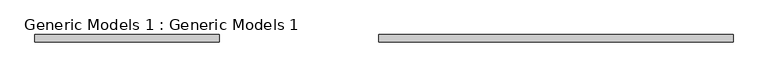
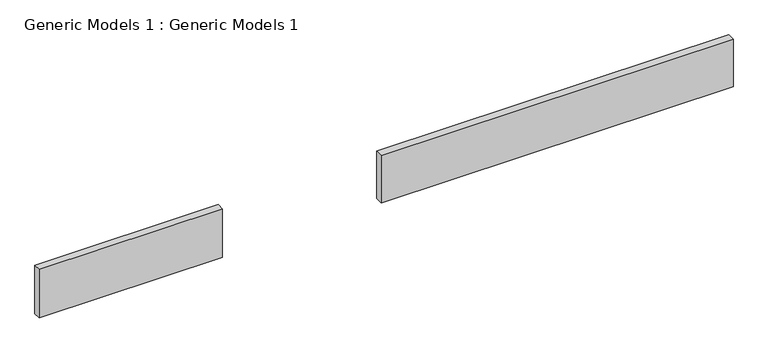
"""IFC4 building model written with IfcOpenShell, lengths in millimetres: proxy geometry, Generic Models 1 : Generic Models 1."""

from ifc_helpers import new_model, si_unit, frame, origin, place, context, project, spatial, polyline, outline, extrude, source, transform, mapped, element, save


def generic_models_1_generic_models_1_70afe8e7(model_context):
    return source(origin(), model_context, "Body", "SweptSolid", [
        extrude(outline(polyline([(6206.1733706, -11533.6232708), (-1109.0266294, -11533.6232708), (-1109.0266294, -11381.2232708), (6206.1733706, -11381.2232708), (6206.1733706, -11533.6232708)])), frame((0.0, 0.0, 258.0789032), z_axis=(0.0, 0.0, 1.0), x_axis=(1.0, 0.0, 0.0)), (0.0, 0.0, 1.0), 1041.2766398),
        extrude(outline(polyline([(-4405.7526885, -11533.6232708), (-8215.7526885, -11533.6232708), (-8215.7526885, -11381.2232708), (-4405.7526885, -11381.2232708), (-4405.7526885, -11533.6232708)])), frame((0.0, 0.0, 212.9612307), z_axis=(0.0, 0.0, 1.0), x_axis=(1.0, 0.0, 0.0)), (0.0, 0.0, 1.0), 1066.8),
    ])


if __name__ == "__main__":
    model = new_model("IFC4")
    model_context = context("Model", 3, world=origin())
    ifc_project = project(units=[si_unit("LENGTHUNIT", "METRE", prefix="MILLI")], contexts=[model_context])
    site = spatial("IfcSite", under=ifc_project)
    building = spatial("IfcBuilding", under=site)
    placement = place(None, origin())
    generic_models_1_generic_models_1_shape = generic_models_1_generic_models_1_70afe8e7(model_context)
    element("IfcBuildingElementProxy", 1, Name="Generic Models 1 : Generic Models 1", ObjectType="Generic Models 1 : Generic Models 1", at=placement, inside=building, context=model_context, shape_type="MappedRepresentation", body=[
        mapped(generic_models_1_generic_models_1_shape, transform((0.0, 0.0, 0.0), x_axis=(1.0, 0.0, 0.0), y_axis=(0.0, 1.0, 0.0), z_axis=(0.0, 0.0, 1.0))),
    ])
    save(model, "model.ifc")

# Revit data of these elements
# Element 1 (IfcBuildingElementProxy, "Generic Models 1 : Generic Models 1")
#   Materials on its faces: "Parking Stripe"
# Materials
#   "Parking Stripe": class "Paint", colour RGB 250 250 91, transparency 0, Cost = 0
